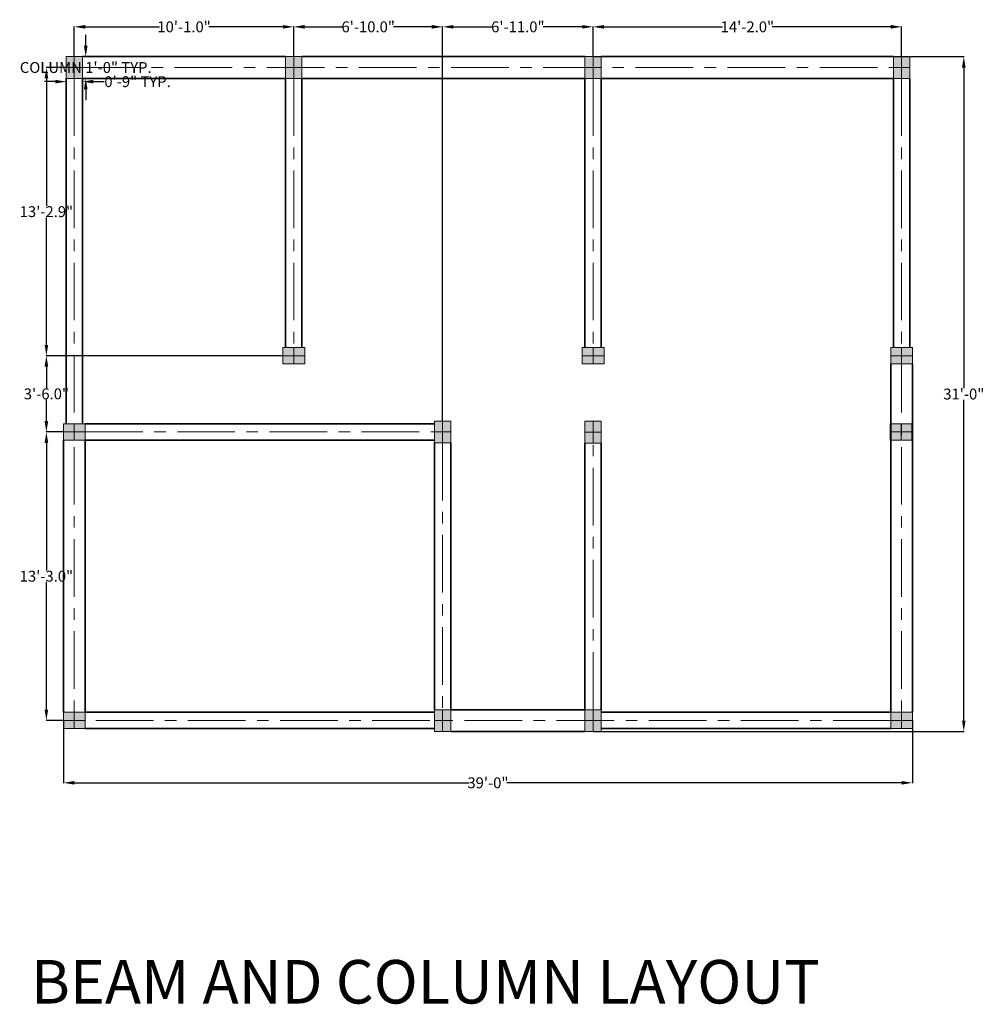
# Model space of a CAD drawing. Units: inches. Extents: x 1966 to 4198, y 2607 to 3884.
# Tile 8 of 8: x 3666 to 4198, y 3133 to 3676. Entities that reach past the tile are written whole.
import ezdxf

# ---------------------------------------------------------------- set-up
doc = ezdxf.new("R2010")
doc.units = ezdxf.units.IN
doc.header["$MEASUREMENT"] = 0
doc.linetypes.add('CENTER', pattern=[50.8, 31.75, -6.35, 6.35, -6.35])
for name, color, linetype, lineweight in [('A-ANNO-TEXT', 4, 'Continuous', 25), ('dimension', 90, 'Continuous', 18), ('furniture', 163, 'Continuous', 18), ('S-BEAM', 163, 'Continuous', 35), ('S-COLS', 163, 'Continuous', 35), ('S-GRID', 163, 'CENTER', 13)]:
    doc.layers.add(name, color=color, linetype=linetype, lineweight=lineweight)
doc.styles.get("Standard").update_dxf_attribs({"font": 'arial.ttf'})
doc.dimstyles.get("Standard").update_dxf_attribs({"dimtxt": 6, "dimasz": 6, "dimexe": 0.18, "dimexo": 0.0625, "dimgap": 0.09, "dimtad": 0, "dimtih": 1, "dimtoh": 1, "dimdec": 1, "dimzin": 0, "dimdsep": 46, "dimlunit": 3, "dimtxsty": 'Standard', "dimcen": 0.09, "dimadec": 0, "dimazin": 0, "dimtfac": 1, "dimtdec": 1, "dimtofl": 0, "dimtmove": 0, "dimatfit": 3, "dimfxl": 1, "dimtolj": 1, "dimtzin": 0, "dimarcsym": 0})

# ---------------------------------------------------------------- blocks, each defined once
blk = doc.blocks.new('COLUMN')
at = {"layer": 'furniture'}
h = blk.add_hatch(color=256, dxfattribs=at)
h.dxf.hatch_style = 1
h.paths.add_polyline_path([(3602.87, 3735.36), (3602.87, 3747.36), (3593.87, 3747.36), (3593.87, 3735.36)])
for p, q in [((3598.37, 3735.36), (3598.37, 3747.36)), ((3593.87, 3741.36), (3602.87, 3741.36))]:
    blk.add_line(p, q, dxfattribs=at)
blk.add_lwpolyline([(3593.87, 3735.36), (3602.87, 3735.36), (3602.87, 3747.36), (3593.87, 3747.36)], close=True, dxfattribs=at)
blk = doc.blocks.new('*D17')
at = {"layer": 'Defpoints', "color": 0, "transparency": 16777216}
for p in [(3680.96, 3448.72), (3690.34, 3448.72), (3690.34, 3289.72)]:
    blk.add_point(p, dxfattribs=at)
at = {"layer": 'dimension', "color": 0, "lineweight": -2, "transparency": 16777216}
for p, q in [((3690.28, 3448.72), (3680.78, 3448.72)), ((3680.96, 3442.72), (3680.96, 3372.38)), ((3680.96, 3295.72), (3680.96, 3366.07)), ((3690.28, 3289.72), (3680.78, 3289.72))]:
    blk.add_line(p, q, dxfattribs=at)
at = {"layer": 'dimension', "color": 0, "transparency": 16777216}
for points in [[(3679.96, 3442.72), (3681.96, 3442.72), (3680.96, 3448.72)], [(3679.96, 3295.72), (3681.96, 3295.72), (3680.96, 3289.72)]]:
    blk.add_solid(points, dxfattribs=at)
at = {"layer": 'dimension', "color": 0, "transparency": 16777216, "insert": (3680.96, 3369.22), "char_height": 6, "attachment_point": 5}
blk.add_mtext('\\A1;13\'-3.0"', dxfattribs=at)
blk = doc.blocks.new('*D18')
at = {"layer": 'Defpoints', "color": 0, "transparency": 16777216}
for p in [(3680.96, 3490.72), (3811.34, 3490.72), (3690.34, 3448.72)]:
    blk.add_point(p, dxfattribs=at)
at = {"layer": 'dimension', "color": 0, "lineweight": -2, "transparency": 16777216}
for p, q in [((3811.28, 3490.72), (3680.78, 3490.72)), ((3680.96, 3484.72), (3680.96, 3472.88)), ((3680.96, 3454.72), (3680.96, 3466.57)), ((3690.28, 3448.72), (3680.78, 3448.72))]:
    blk.add_line(p, q, dxfattribs=at)
at = {"layer": 'dimension', "color": 0, "transparency": 16777216}
for points in [[(3679.96, 3484.72), (3681.96, 3484.72), (3680.96, 3490.72)], [(3679.96, 3454.72), (3681.96, 3454.72), (3680.96, 3448.72)]]:
    blk.add_solid(points, dxfattribs=at)
at = {"layer": 'dimension', "color": 0, "transparency": 16777216, "insert": (3680.96, 3469.72), "char_height": 6, "attachment_point": 5}
blk.add_mtext('\\A1;3\'-6.0"', dxfattribs=at)
blk = doc.blocks.new('*D19')
at = {"layer": 'Defpoints', "color": 0, "transparency": 16777216}
for p in [(3680.96, 3649.62), (3691.84, 3649.62), (3811.34, 3490.72)]:
    blk.add_point(p, dxfattribs=at)
at = {"layer": 'dimension', "color": 0, "lineweight": -2, "transparency": 16777216}
for p, q in [((3691.78, 3649.62), (3680.78, 3649.62)), ((3680.96, 3643.62), (3680.96, 3573.32)), ((3680.96, 3496.72), (3680.96, 3567.01)), ((3811.28, 3490.72), (3680.78, 3490.72))]:
    blk.add_line(p, q, dxfattribs=at)
at = {"layer": 'dimension', "color": 0, "transparency": 16777216}
for points in [[(3679.96, 3643.62), (3681.96, 3643.62), (3680.96, 3649.62)], [(3679.96, 3496.72), (3681.96, 3496.72), (3680.96, 3490.72)]]:
    blk.add_solid(points, dxfattribs=at)
at = {"layer": 'dimension', "color": 0, "transparency": 16777216, "insert": (3680.96, 3570.17), "char_height": 6, "attachment_point": 5}
blk.add_mtext('\\A1;13\'-2.9"', dxfattribs=at)
blk = doc.blocks.new('*D20')
at = {"layer": 'Defpoints', "color": 0, "transparency": 16777216}
for p in [(3817.34, 3672.04), (3696.34, 3655.62), (3817.34, 3655.62)]:
    blk.add_point(p, dxfattribs=at)
at = {"layer": 'dimension', "color": 0, "lineweight": -2, "transparency": 16777216}
for p, q in [((3696.34, 3655.68), (3696.34, 3672.22)), ((3702.34, 3672.04), (3743.23, 3672.04)), ((3811.34, 3672.04), (3770.45, 3672.04)), ((3817.34, 3655.68), (3817.34, 3672.22))]:
    blk.add_line(p, q, dxfattribs=at)
at = {"layer": 'dimension', "color": 0, "transparency": 16777216}
for points in [[(3702.34, 3673.04), (3702.34, 3671.04), (3696.34, 3672.04)], [(3811.34, 3673.04), (3811.34, 3671.04), (3817.34, 3672.04)]]:
    blk.add_solid(points, dxfattribs=at)
at = {"layer": 'dimension', "color": 0, "transparency": 16777216, "insert": (3756.84, 3672.04), "char_height": 6, "attachment_point": 5}
blk.add_mtext('\\A1;10\'-1.0"', dxfattribs=at)
blk = doc.blocks.new('*D21')
at = {"layer": 'Defpoints', "color": 0, "transparency": 16777216}
for p in [(3899.34, 3672.04), (3817.34, 3655.62), (3899.34, 3454.72)]:
    blk.add_point(p, dxfattribs=at)
at = {"layer": 'dimension', "color": 0, "lineweight": -2, "transparency": 16777216}
for p, q in [((3817.34, 3655.68), (3817.34, 3672.22)), ((3823.34, 3672.04), (3844.43, 3672.04)), ((3893.34, 3672.04), (3872.25, 3672.04)), ((3899.34, 3454.78), (3899.34, 3672.22))]:
    blk.add_line(p, q, dxfattribs=at)
at = {"layer": 'dimension', "color": 0, "transparency": 16777216}
for points in [[(3823.34, 3673.04), (3823.34, 3671.04), (3817.34, 3672.04)], [(3893.34, 3673.04), (3893.34, 3671.04), (3899.34, 3672.04)]]:
    blk.add_solid(points, dxfattribs=at)
at = {"layer": 'dimension', "color": 0, "transparency": 16777216, "insert": (3858.34, 3672.04), "char_height": 6, "attachment_point": 5}
blk.add_mtext('\\A1;6\'-10.0"', dxfattribs=at)
blk = doc.blocks.new('*D22')
at = {"layer": 'Defpoints', "color": 0, "transparency": 16777216}
for p in [(3982.34, 3672.04), (3982.34, 3655.62), (3899.34, 3454.72)]:
    blk.add_point(p, dxfattribs=at)
at = {"layer": 'dimension', "color": 0, "lineweight": -2, "transparency": 16777216}
for p, q in [((3899.34, 3454.78), (3899.34, 3672.22)), ((3905.34, 3672.04), (3926.93, 3672.04)), ((3976.34, 3672.04), (3954.75, 3672.04)), ((3982.34, 3655.68), (3982.34, 3672.22))]:
    blk.add_line(p, q, dxfattribs=at)
at = {"layer": 'dimension', "color": 0, "transparency": 16777216}
for points in [[(3905.34, 3673.04), (3905.34, 3671.04), (3899.34, 3672.04)], [(3976.34, 3673.04), (3976.34, 3671.04), (3982.34, 3672.04)]]:
    blk.add_solid(points, dxfattribs=at)
at = {"layer": 'dimension', "color": 0, "transparency": 16777216, "insert": (3940.84, 3672.04), "char_height": 6, "attachment_point": 5}
blk.add_mtext('\\A1;6\'-11.0"', dxfattribs=at)
blk = doc.blocks.new('*D23')
at = {"layer": 'Defpoints', "color": 0, "transparency": 16777216}
for p in [(4152.34, 3672.04), (3982.34, 3655.62), (4152.34, 3655.62)]:
    blk.add_point(p, dxfattribs=at)
at = {"layer": 'dimension', "color": 0, "lineweight": -2, "transparency": 16777216}
for p, q in [((3982.34, 3655.68), (3982.34, 3672.22)), ((3988.34, 3672.04), (4053.73, 3672.04)), ((4146.34, 3672.04), (4080.95, 3672.04)), ((4152.34, 3655.68), (4152.34, 3672.22))]:
    blk.add_line(p, q, dxfattribs=at)
at = {"layer": 'dimension', "color": 0, "transparency": 16777216}
for points in [[(3988.34, 3673.04), (3988.34, 3671.04), (3982.34, 3672.04)], [(4146.34, 3673.04), (4146.34, 3671.04), (4152.34, 3672.04)]]:
    blk.add_solid(points, dxfattribs=at)
at = {"layer": 'dimension', "color": 0, "transparency": 16777216, "insert": (4067.34, 3672.04), "char_height": 6, "attachment_point": 5}
blk.add_mtext('\\A1;14\'-2.0"', dxfattribs=at)
blk = doc.blocks.new('*D41')
at = {"layer": 'Defpoints', "color": 0, "transparency": 16777216}
for p in [(3700.84, 3655.62), (3702.64, 3655.62), (3700.84, 3643.62)]:
    blk.add_point(p, dxfattribs=at)
at = {"layer": 'dimension', "color": 0, "lineweight": -2, "transparency": 16777216}
for p, q in [((3702.64, 3661.62), (3702.64, 3667.62)), ((3700.9, 3655.62), (3702.82, 3655.62)), ((3700.9, 3643.62), (3702.82, 3643.62)), ((3702.64, 3637.62), (3702.64, 3631.62))]:
    blk.add_line(p, q, dxfattribs=at)
at = {"layer": 'dimension', "color": 0, "transparency": 16777216}
for points in [[(3701.64, 3661.62), (3703.64, 3661.62), (3702.64, 3655.62)], [(3701.64, 3637.62), (3703.64, 3637.62), (3702.64, 3643.62)]]:
    blk.add_solid(points, dxfattribs=at)
at = {"layer": 'dimension', "color": 0, "transparency": 16777216, "insert": (3702.64, 3649.62), "char_height": 6, "attachment_point": 5}
blk.add_mtext('\\A1;COLUMN 1\'-0" TYP.', dxfattribs=at)
blk = doc.blocks.new('*D42')
at = {"layer": 'Defpoints', "color": 0, "transparency": 16777216}
for p in [(3691.84, 3643.62), (3700.84, 3643.62), (3700.84, 3641.82)]:
    blk.add_point(p, dxfattribs=at)
at = {"layer": 'dimension', "color": 0, "lineweight": -2, "transparency": 16777216}
for p, q in [((3691.84, 3643.56), (3691.84, 3641.64)), ((3700.84, 3643.56), (3700.84, 3641.64)), ((3685.84, 3641.82), (3679.84, 3641.82)), ((3706.84, 3641.82), (3712.84, 3641.82))]:
    blk.add_line(p, q, dxfattribs=at)
at = {"layer": 'dimension', "color": 0, "transparency": 16777216}
for points in [[(3685.84, 3642.82), (3685.84, 3640.82), (3691.84, 3641.82)], [(3706.84, 3642.82), (3706.84, 3640.82), (3700.84, 3641.82)]]:
    blk.add_solid(points, dxfattribs=at)
at = {"layer": 'dimension', "color": 0, "transparency": 16777216, "insert": (3731.22, 3641.82), "char_height": 6, "attachment_point": 5}
blk.add_mtext('\\A1;0\'-9" TYP.', dxfattribs=at)
blk = doc.blocks.new('*D100')
at = {"layer": 'Defpoints', "color": 0, "transparency": 16777216}
for p in [(3690.34, 3289.72), (4158.34, 3289.72), (4158.34, 3255.32)]:
    blk.add_point(p, dxfattribs=at)
at = {"layer": 'dimension', "color": 0, "lineweight": -2, "transparency": 16777216}
for p, q in [((3690.34, 3289.66), (3690.34, 3255.14)), ((4158.34, 3289.66), (4158.34, 3255.14)), ((3696.34, 3255.32), (3913.95, 3255.32)), ((4152.34, 3255.32), (3934.73, 3255.32))]:
    blk.add_line(p, q, dxfattribs=at)
at = {"layer": 'dimension', "color": 0, "transparency": 16777216}
for points in [[(3696.34, 3256.32), (3696.34, 3254.32), (3690.34, 3255.32)], [(4152.34, 3256.32), (4152.34, 3254.32), (4158.34, 3255.32)]]:
    blk.add_solid(points, dxfattribs=at)
at = {"layer": 'dimension', "color": 0, "transparency": 16777216, "insert": (3924.34, 3255.32), "char_height": 6, "attachment_point": 5}
blk.add_mtext('\\A1;39\'-0"', dxfattribs=at)
blk = doc.blocks.new('*D101')
at = {"layer": 'Defpoints', "color": 0, "transparency": 16777216}
for p in [(3982.34, 3655.62), (4186.64, 3655.62), (3982.34, 3283.62)]:
    blk.add_point(p, dxfattribs=at)
at = {"layer": 'dimension', "color": 0, "lineweight": -2, "transparency": 16777216}
for p, q in [((3982.4, 3655.62), (4186.82, 3655.62)), ((4186.64, 3649.62), (4186.64, 3472.77)), ((4186.64, 3289.62), (4186.64, 3466.46)), ((3982.4, 3283.62), (4186.82, 3283.62))]:
    blk.add_line(p, q, dxfattribs=at)
at = {"layer": 'dimension', "color": 0, "transparency": 16777216}
for points in [[(4185.64, 3649.62), (4187.64, 3649.62), (4186.64, 3655.62)], [(4185.64, 3289.62), (4187.64, 3289.62), (4186.64, 3283.62)]]:
    blk.add_solid(points, dxfattribs=at)
at = {"layer": 'dimension', "color": 0, "transparency": 16777216, "insert": (4186.64, 3469.62), "char_height": 6, "attachment_point": 5}
blk.add_mtext('\\A1;31\'-0"', dxfattribs=at)

msp = doc.modelspace()

# ---------------------------------------------------------------- linework, layer by layer
at = {"layer": 'S-BEAM'}
for p, q in [((3700.84, 3655.62), (3812.84, 3655.62)), ((3821.84, 3655.62), (3977.84, 3655.62)), ((3986.84, 3655.62), (4147.84, 3655.62)), ((3691.84, 3643.62), (3691.84, 3453.22)), ((3700.84, 3643.62), (3812.84, 3643.62)), ((3700.84, 3643.62), (3700.84, 3453.22)), ((3812.84, 3643.62), (3812.84, 3495.22)), ((3821.84, 3643.62), (3977.84, 3643.62)), ((3821.84, 3643.62), (3821.84, 3495.22)), ((3977.84, 3643.62), (3977.84, 3495.22)), ((3986.84, 3643.62), (4147.84, 3643.62)), ((3986.84, 3643.62), (3986.84, 3495.22)), ((4147.84, 3643.62), (4147.84, 3495.22)), ((4156.84, 3643.62), (4156.84, 3495.22)), ((4146.34, 3486.22), (4146.34, 3294.22)), ((4158.34, 3294.22), (4158.34, 3486.22)), ((3702.34, 3453.22), (3894.84, 3453.22)), ((3690.34, 3294.22), (3690.34, 3444.22)), ((3702.34, 3444.22), (3702.34, 3294.22)), ((3702.34, 3444.22), (3894.84, 3444.22)), ((3894.84, 3442.72), (3894.84, 3295.62)), ((3903.84, 3442.72), (3903.84, 3295.62)), ((3977.84, 3442.62), (3977.84, 3295.62)), ((3986.84, 3442.62), (3986.84, 3295.62)), ((3903.84, 3295.62), (3977.84, 3295.62)), ((3702.34, 3294.22), (3894.84, 3294.22)), ((4146.34, 3294.22), (3986.84, 3294.22)), ((3702.34, 3285.22), (3894.84, 3285.22)), ((4146.34, 3285.22), (3986.84, 3285.22)), ((3903.84, 3283.62), (3977.84, 3283.62))]:
    msp.add_line(p, q, dxfattribs=at)
at = {"layer": 'S-GRID'}
for p, q in [((3700.84, 3649.62), (4147.84, 3649.62)), ((3696.34, 3643.62), (3696.34, 3294.22)), ((3817.34, 3643.62), (3817.34, 3495.22)), ((3982.34, 3643.62), (3982.34, 3495.22)), ((4152.34, 3643.62), (4152.34, 3294.22)), ((3702.34, 3448.72), (3894.84, 3448.72)), ((3899.34, 3442.72), (3899.34, 3295.62)), ((3982.34, 3295.62), (3982.34, 3442.62)), ((4146.34, 3289.72), (3702.34, 3289.72))]:
    msp.add_line(p, q, dxfattribs=at)

# ---------------------------------------------------------------- block references
at = {"layer": 'S-COLS'}
for p in [(97.97, -91.75), (218.97, -91.75), (383.97, -91.75), (553.97, -91.75), (300.97, -292.64), (383.97, -292.75), (300.97, -451.75), (383.97, -451.75)]:
    msp.add_blockref('COLUMN', p, dxfattribs=at)
at = {"layer": 'S-COLS', "rotation": 90}
for p in [(7558.7, -107.65), (7723.7, -107.65), (7893.7, -107.65), (7437.7, -149.65), (7893.43, -149.65), (7437.7, -308.65), (7893.7, -308.65)]:
    msp.add_blockref('COLUMN', p, dxfattribs=at)

# ---------------------------------------------------------------- texts
at = {"layer": 'A-ANNO-TEXT', "insert": (3889.84, 3157.64), "char_height": 24, "attachment_point": 2}
msp.add_mtext_dynamic_manual_height_columns('BEAM AND COLUMN LAYOUT', width=566.4905, gutter_width=1, heights=[0], dxfattribs=at)

# ---------------------------------------------------------------- dimensions: what is measured, and where the dimension line sits
at = {"layer": 'dimension'}
for base, p1, p2, override, picture, middle in [((3817.34, 3672.04), (3696.34, 3655.62), (3817.34, 3655.62), {"dimclrd": 0, "dimclre": 0, "dimclrt": 0}, '*D20', (3756.84, 3672.04)), ((3899.34, 3672.04), (3817.34, 3655.62), (3899.34, 3454.72), {"dimclrd": 0, "dimclre": 0, "dimclrt": 0, "dimtmove": 1}, '*D21', (3858.34, 3672.04)), ((3982.34, 3672.04), (3899.34, 3454.72), (3982.34, 3655.62), {"dimclrd": 0, "dimclre": 0, "dimclrt": 0, "dimtmove": 1}, '*D22', (3940.84, 3672.04)), ((4152.34, 3672.04), (3982.34, 3655.62), (4152.34, 3655.62), {"dimclrd": 0, "dimclre": 0, "dimclrt": 0, "dimtmove": 1}, '*D23', (4067.34, 3672.04)), ((4158.34, 3255.32), (3690.34, 3289.72), (4158.34, 3289.72), {"dimdec": 1, "dimlfac": 1, "dimrnd": 0, "dimzin": 1, "dimdsep": 46, "dimlunit": 4, "dimfrac": 2}, '*D100', (3924.34, 3255.32))]:
    dim = msp.add_linear_dim(base=base, p1=p1, p2=p2, dimstyle='Standard', override=override, dxfattribs=at)
    dim.commit()
    dim.dimension.update_dxf_attribs({"geometry": picture, "text_midpoint": middle})
dim = msp.add_linear_dim(base=(3702.64, 3655.62), p1=(3700.84, 3643.62), p2=(3700.84, 3655.62), angle=90, text='COLUMN <> TYP.', dimstyle='Standard', override={"dimdec": 1, "dimlfac": 1, "dimrnd": 0, "dimzin": 1, "dimdsep": 46, "dimlunit": 4, "dimfrac": 2}, dxfattribs=at)
dim.commit()
dim.dimension.update_dxf_attribs({"geometry": '*D41', "text_midpoint": (3702.64, 3649.62)})
for base, p1, p2, override, picture, middle in [((4186.64, 3655.62), (3982.34, 3283.62), (3982.34, 3655.62), {"dimdec": 1, "dimlfac": 1, "dimrnd": 0, "dimzin": 1, "dimdsep": 46, "dimlunit": 4, "dimfrac": 2}, '*D101', (4186.64, 3469.62)), ((3680.96, 3649.62), (3811.34, 3490.72), (3691.84, 3649.62), {"dimclrd": 0, "dimclre": 0, "dimclrt": 0, "dimtmove": 1}, '*D19', (3680.96, 3570.17)), ((3680.96, 3490.72), (3690.34, 3448.72), (3811.34, 3490.72), {"dimclrd": 0, "dimclre": 0, "dimclrt": 0, "dimtmove": 1}, '*D18', (3680.96, 3469.72)), ((3680.96, 3448.72), (3690.34, 3289.72), (3690.34, 3448.72), {"dimclrd": 0, "dimclre": 0, "dimclrt": 0}, '*D17', (3680.96, 3369.22))]:
    dim = msp.add_linear_dim(base=base, p1=p1, p2=p2, angle=90, dimstyle='Standard', override=override, dxfattribs=at)
    dim.commit()
    dim.dimension.update_dxf_attribs({"geometry": picture, "text_midpoint": middle})
dim = msp.add_linear_dim(base=(3700.84, 3641.82), p1=(3691.84, 3643.62), p2=(3700.84, 3643.62), text='<> TYP.', dimstyle='Standard', override={"dimdec": 1, "dimlfac": 1, "dimrnd": 0, "dimzin": 1, "dimdsep": 46, "dimlunit": 4, "dimfrac": 2}, dxfattribs=at)
dim.commit()
dim.dimension.update_dxf_attribs({"geometry": '*D42', "text_midpoint": (3731.22, 3641.82)})

doc.saveas('drawing.dxf')
